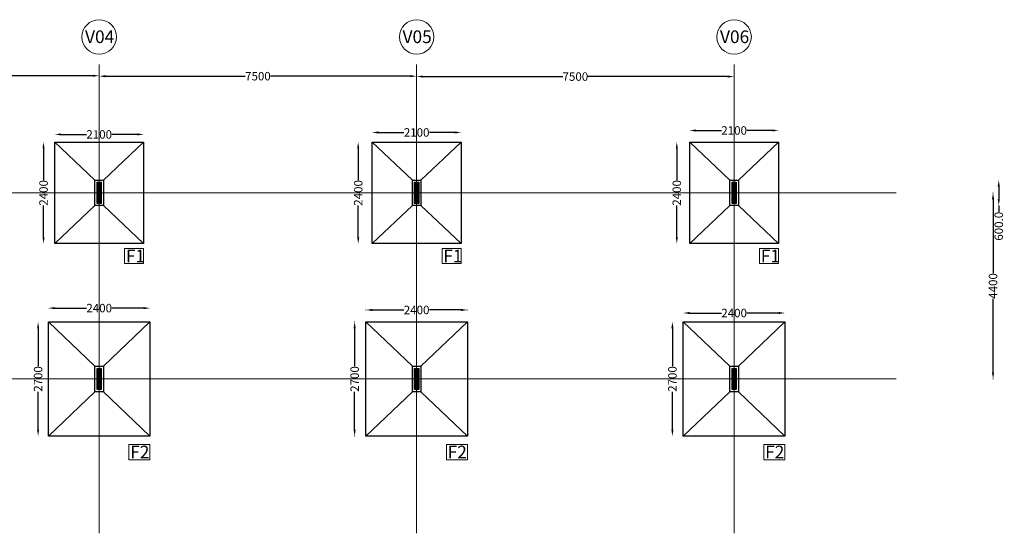
# Model space of a CAD drawing. Units: millimetres. Extents: x -30630 to 20484, y 3580 to 30715.
# Tile 4 of 4: x -3358 to 19903, y 16016 to 28161. Entities that reach past the tile are written whole.
import ezdxf

# ---------------------------------------------------------------- set-up
doc = ezdxf.new("R2010")
doc.units = ezdxf.units.MM
doc.header["$MEASUREMENT"] = 0
for name, color, linetype, lineweight in [('S-ANNO-DIMS', 2, 'Continuous', 18), ('S-ANNO-SYMB', 3, 'Continuous', 18), ('S-ANNO-TEXT', 7, 'Continuous', 18), ('S-FNDN', 7, 'Continuous', 30), ('S-GRID', 1, 'Continuous', 18), ('S-GRID-IDEN', 7, 'Continuous', 18)]:
    doc.layers.add(name, color=color, linetype=linetype, lineweight=lineweight)
doc.styles.get("Standard").update_dxf_attribs({"font": 'arial.ttf'})
doc.dimstyles.get("Standard").update_dxf_attribs({"dimtxt": 200, "dimasz": 150, "dimexe": 0.18, "dimexo": 0.0625, "dimgap": 0.09, "dimtad": 0, "dimdec": 0, "dimzin": 0, "dimdsep": 46, "dimtxsty": 'Standard', "dimcen": 0.09, "dimadec": 0, "dimazin": 0, "dimtfac": 1, "dimtdec": 0, "dimtofl": 0, "dimtmove": 0, "dimatfit": 3, "dimfxl": 1, "dimfxlon": 1, "dimtolj": 1, "dimtzin": 0, "dimarcsym": 0})

# ---------------------------------------------------------------- blocks, each defined once
blk = doc.blocks.new('*D5')
at = {"layer": 'Defpoints', "color": 0, "transparency": 16777216}
for p in [(-8980, 26835), (-8980, 26552), (-1480, 26552)]:
    blk.add_point(p, dxfattribs=at)
at = {"layer": 'S-ANNO-DIMS', "color": 0, "lineweight": -2, "transparency": 16777216}
for p, q in [((-8980, 26834), (-8980, 26836)), ((-8830, 26835), (-5528, 26835)), ((-1630, 26835), (-4933, 26835)), ((-1480, 26834), (-1480, 26836))]:
    blk.add_line(p, q, dxfattribs=at)
at = {"layer": 'S-ANNO-DIMS', "color": 0, "transparency": 16777216}
for points in [[(-8830, 26860), (-8830, 26810), (-8980, 26835)], [(-1630, 26860), (-1630, 26810), (-1480, 26835)]]:
    blk.add_solid(points, dxfattribs=at)
at = {"layer": 'S-ANNO-DIMS', "color": 0, "transparency": 16777216, "insert": (-5230, 26835), "char_height": 200, "attachment_point": 5}
blk.add_mtext('\\A1;7500', dxfattribs=at)
blk = doc.blocks.new('*D6')
at = {"layer": 'Defpoints', "color": 0, "transparency": 16777216}
for p in [(-1480, 26825), (-1480, 26456), (6020, 26456)]:
    blk.add_point(p, dxfattribs=at)
at = {"layer": 'S-ANNO-DIMS', "color": 0, "lineweight": -2, "transparency": 16777216}
for p, q in [((-1480, 26824), (-1480, 26825)), ((-1330, 26825), (1972, 26825)), ((5870, 26825), (2567, 26825)), ((6020, 26824), (6020, 26825))]:
    blk.add_line(p, q, dxfattribs=at)
at = {"layer": 'S-ANNO-DIMS', "color": 0, "transparency": 16777216}
for points in [[(-1330, 26850), (-1330, 26800), (-1480, 26825)], [(5870, 26850), (5870, 26800), (6020, 26825)]]:
    blk.add_solid(points, dxfattribs=at)
at = {"layer": 'S-ANNO-DIMS', "color": 0, "transparency": 16777216, "insert": (2270, 26825), "char_height": 200, "attachment_point": 5}
blk.add_mtext('\\A1;7500', dxfattribs=at)
blk = doc.blocks.new('*D7')
at = {"layer": 'Defpoints', "color": 0, "transparency": 16777216}
for p in [(6020, 26816), (6020, 26492), (13520, 26492)]:
    blk.add_point(p, dxfattribs=at)
at = {"layer": 'S-ANNO-DIMS', "color": 0, "lineweight": -2, "transparency": 16777216}
for p, q in [((6020, 26815), (6020, 26816)), ((6170, 26816), (9472, 26816)), ((13370, 26816), (10067, 26816)), ((13520, 26815), (13520, 26816))]:
    blk.add_line(p, q, dxfattribs=at)
at = {"layer": 'S-ANNO-DIMS', "color": 0, "transparency": 16777216}
for points in [[(6170, 26841), (6170, 26791), (6020, 26816)], [(13370, 26841), (13370, 26791), (13520, 26816)]]:
    blk.add_solid(points, dxfattribs=at)
at = {"layer": 'S-ANNO-DIMS', "color": 0, "transparency": 16777216, "insert": (9770, 26816), "char_height": 200, "attachment_point": 5}
blk.add_mtext('\\A1;7500', dxfattribs=at)
blk = doc.blocks.new('*D14')
at = {"layer": 'Defpoints', "color": 0, "transparency": 16777216}
for p in [(-2530, 25448), (-2530, 25265), (-430, 25265)]:
    blk.add_point(p, dxfattribs=at)
at = {"layer": 'S-ANNO-DIMS', "color": 0, "lineweight": -2, "transparency": 16777216}
for p, q in [((-2530, 25447), (-2530, 25448)), ((-2380, 25448), (-1780, 25448)), ((-580, 25448), (-1180, 25448)), ((-430, 25447), (-430, 25448))]:
    blk.add_line(p, q, dxfattribs=at)
at = {"layer": 'S-ANNO-DIMS', "color": 0, "transparency": 16777216}
for points in [[(-2380, 25473), (-2380, 25423), (-2530, 25448)], [(-580, 25473), (-580, 25423), (-430, 25448)]]:
    blk.add_solid(points, dxfattribs=at)
at = {"layer": 'S-ANNO-DIMS', "color": 0, "transparency": 16777216, "insert": (-1480, 25448), "char_height": 200, "attachment_point": 5}
blk.add_mtext('\\A1;2100', dxfattribs=at)
blk = doc.blocks.new('*D15')
at = {"layer": 'Defpoints', "color": 0, "transparency": 16777216}
for p in [(-2530, 25265), (-2795, 22865), (-2530, 22865)]:
    blk.add_point(p, dxfattribs=at)
at = {"layer": 'S-ANNO-DIMS', "color": 0, "lineweight": -2, "transparency": 16777216}
for p, q in [((-2794, 25265), (-2795, 25265)), ((-2795, 25115), (-2795, 24365)), ((-2795, 23015), (-2795, 23765)), ((-2794, 22865), (-2795, 22865))]:
    blk.add_line(p, q, dxfattribs=at)
at = {"layer": 'S-ANNO-DIMS', "color": 0, "transparency": 16777216}
for points in [[(-2820, 25115), (-2770, 25115), (-2795, 25265)], [(-2820, 23015), (-2770, 23015), (-2795, 22865)]]:
    blk.add_solid(points, dxfattribs=at)
at = {"layer": 'S-ANNO-DIMS', "color": 0, "transparency": 16777216, "insert": (-2795, 24065), "char_height": 200, "attachment_point": 5, "rotation": 90}
blk.add_mtext('\\A1;2400', dxfattribs=at)
blk = doc.blocks.new('*D16')
at = {"layer": 'Defpoints', "color": 0, "transparency": 16777216}
for p in [(7070, 25494), (4970, 25265), (7070, 25265)]:
    blk.add_point(p, dxfattribs=at)
at = {"layer": 'S-ANNO-DIMS', "color": 0, "lineweight": -2, "transparency": 16777216}
for p, q in [((4970, 25493), (4970, 25495)), ((5120, 25494), (5720, 25494)), ((6920, 25494), (6320, 25494)), ((7070, 25493), (7070, 25495))]:
    blk.add_line(p, q, dxfattribs=at)
at = {"layer": 'S-ANNO-DIMS', "color": 0, "transparency": 16777216}
for points in [[(5120, 25519), (5120, 25469), (4970, 25494)], [(6920, 25519), (6920, 25469), (7070, 25494)]]:
    blk.add_solid(points, dxfattribs=at)
at = {"layer": 'S-ANNO-DIMS', "color": 0, "transparency": 16777216, "insert": (6020, 25494), "char_height": 200, "attachment_point": 5}
blk.add_mtext('\\A1;2100', dxfattribs=at)
blk = doc.blocks.new('*D17')
at = {"layer": 'Defpoints', "color": 0, "transparency": 16777216}
for p in [(4970, 25265), (4639, 22865), (4970, 22865)]:
    blk.add_point(p, dxfattribs=at)
at = {"layer": 'S-ANNO-DIMS', "color": 0, "lineweight": -2, "transparency": 16777216}
for p, q in [((4640, 25265), (4639, 25265)), ((4639, 25115), (4639, 24365)), ((4639, 23015), (4639, 23765)), ((4640, 22865), (4639, 22865))]:
    blk.add_line(p, q, dxfattribs=at)
at = {"layer": 'S-ANNO-DIMS', "color": 0, "transparency": 16777216}
for points in [[(4614, 25115), (4664, 25115), (4639, 25265)], [(4614, 23015), (4664, 23015), (4639, 22865)]]:
    blk.add_solid(points, dxfattribs=at)
at = {"layer": 'S-ANNO-DIMS', "color": 0, "transparency": 16777216, "insert": (4639, 24065), "char_height": 200, "attachment_point": 5, "rotation": 90}
blk.add_mtext('\\A1;2400', dxfattribs=at)
blk = doc.blocks.new('*D18')
at = {"layer": 'Defpoints', "color": 0, "transparency": 16777216}
for p in [(12470, 25541), (12470, 25265), (14570, 25265)]:
    blk.add_point(p, dxfattribs=at)
at = {"layer": 'S-ANNO-DIMS', "color": 0, "lineweight": -2, "transparency": 16777216}
for p, q in [((12470, 25540), (12470, 25542)), ((12620, 25541), (13220, 25541)), ((14420, 25541), (13820, 25541)), ((14570, 25540), (14570, 25542))]:
    blk.add_line(p, q, dxfattribs=at)
at = {"layer": 'S-ANNO-DIMS', "color": 0, "transparency": 16777216}
for points in [[(12620, 25566), (12620, 25516), (12470, 25541)], [(14420, 25566), (14420, 25516), (14570, 25541)]]:
    blk.add_solid(points, dxfattribs=at)
at = {"layer": 'S-ANNO-DIMS', "color": 0, "transparency": 16777216, "insert": (13520, 25541), "char_height": 200, "attachment_point": 5}
blk.add_mtext('\\A1;2100', dxfattribs=at)
blk = doc.blocks.new('*D19')
at = {"layer": 'Defpoints', "color": 0, "transparency": 16777216}
for p in [(12470, 25265), (12166, 22865), (12470, 22865)]:
    blk.add_point(p, dxfattribs=at)
at = {"layer": 'S-ANNO-DIMS', "color": 0, "lineweight": -2, "transparency": 16777216}
for p, q in [((12167, 25265), (12166, 25265)), ((12166, 25115), (12166, 24365)), ((12166, 23015), (12166, 23765)), ((12167, 22865), (12166, 22865))]:
    blk.add_line(p, q, dxfattribs=at)
at = {"layer": 'S-ANNO-DIMS', "color": 0, "transparency": 16777216}
for points in [[(12141, 25115), (12191, 25115), (12166, 25265)], [(12141, 23015), (12191, 23015), (12166, 22865)]]:
    blk.add_solid(points, dxfattribs=at)
at = {"layer": 'S-ANNO-DIMS', "color": 0, "transparency": 16777216, "insert": (12166, 24065), "char_height": 200, "attachment_point": 5, "rotation": 90}
blk.add_mtext('\\A1;2400', dxfattribs=at)
blk = doc.blocks.new('*D26')
at = {"layer": 'Defpoints', "color": 0, "transparency": 16777216}
for p in [(-2680, 21341), (-2680, 21015), (-280, 21015)]:
    blk.add_point(p, dxfattribs=at)
at = {"layer": 'S-ANNO-DIMS', "color": 0, "lineweight": -2, "transparency": 16777216}
for p, q in [((-2680, 21340), (-2680, 21341)), ((-2530, 21341), (-1780, 21341)), ((-430, 21341), (-1180, 21341)), ((-280, 21340), (-280, 21341))]:
    blk.add_line(p, q, dxfattribs=at)
at = {"layer": 'S-ANNO-DIMS', "color": 0, "transparency": 16777216}
for points in [[(-2530, 21366), (-2530, 21316), (-2680, 21341)], [(-430, 21366), (-430, 21316), (-280, 21341)]]:
    blk.add_solid(points, dxfattribs=at)
at = {"layer": 'S-ANNO-DIMS', "color": 0, "transparency": 16777216, "insert": (-1480, 21341), "char_height": 200, "attachment_point": 5}
blk.add_mtext('\\A1;2400', dxfattribs=at)
blk = doc.blocks.new('*D27')
at = {"layer": 'Defpoints', "color": 0, "transparency": 16777216}
for p in [(-2680, 21015), (-2923, 18315), (-2680, 18315)]:
    blk.add_point(p, dxfattribs=at)
at = {"layer": 'S-ANNO-DIMS', "color": 0, "lineweight": -2, "transparency": 16777216}
for p, q in [((-2922, 21015), (-2923, 21015)), ((-2923, 20865), (-2923, 19965)), ((-2923, 18465), (-2923, 19365)), ((-2922, 18315), (-2923, 18315))]:
    blk.add_line(p, q, dxfattribs=at)
at = {"layer": 'S-ANNO-DIMS', "color": 0, "transparency": 16777216}
for points in [[(-2948, 20865), (-2898, 20865), (-2923, 21015)], [(-2948, 18465), (-2898, 18465), (-2923, 18315)]]:
    blk.add_solid(points, dxfattribs=at)
at = {"layer": 'S-ANNO-DIMS', "color": 0, "transparency": 16777216, "insert": (-2923, 19665), "char_height": 200, "attachment_point": 5, "rotation": 90}
blk.add_mtext('\\A1;2700', dxfattribs=at)
blk = doc.blocks.new('*D28')
at = {"layer": 'Defpoints', "color": 0, "transparency": 16777216}
for p in [(4820, 21297), (4820, 21015), (7220, 21015)]:
    blk.add_point(p, dxfattribs=at)
at = {"layer": 'S-ANNO-DIMS', "color": 0, "lineweight": -2, "transparency": 16777216}
for p, q in [((4820, 21296), (4820, 21298)), ((4970, 21297), (5720, 21297)), ((7070, 21297), (6320, 21297)), ((7220, 21296), (7220, 21298))]:
    blk.add_line(p, q, dxfattribs=at)
at = {"layer": 'S-ANNO-DIMS', "color": 0, "transparency": 16777216}
for points in [[(4970, 21322), (4970, 21272), (4820, 21297)], [(7070, 21322), (7070, 21272), (7220, 21297)]]:
    blk.add_solid(points, dxfattribs=at)
at = {"layer": 'S-ANNO-DIMS', "color": 0, "transparency": 16777216, "insert": (6020, 21297), "char_height": 200, "attachment_point": 5}
blk.add_mtext('\\A1;2400', dxfattribs=at)
blk = doc.blocks.new('*D29')
at = {"layer": 'Defpoints', "color": 0, "transparency": 16777216}
for p in [(4820, 21015), (4555, 18315), (4820, 18315)]:
    blk.add_point(p, dxfattribs=at)
at = {"layer": 'S-ANNO-DIMS', "color": 0, "lineweight": -2, "transparency": 16777216}
for p, q in [((4556, 21015), (4555, 21015)), ((4555, 20865), (4555, 19965)), ((4555, 18465), (4555, 19365)), ((4556, 18315), (4555, 18315))]:
    blk.add_line(p, q, dxfattribs=at)
at = {"layer": 'S-ANNO-DIMS', "color": 0, "transparency": 16777216}
for points in [[(4530, 20865), (4580, 20865), (4555, 21015)], [(4530, 18465), (4580, 18465), (4555, 18315)]]:
    blk.add_solid(points, dxfattribs=at)
at = {"layer": 'S-ANNO-DIMS', "color": 0, "transparency": 16777216, "insert": (4555, 19665), "char_height": 200, "attachment_point": 5, "rotation": 90}
blk.add_mtext('\\A1;2700', dxfattribs=at)
blk = doc.blocks.new('*D30')
at = {"layer": 'Defpoints', "color": 0, "transparency": 16777216}
for p in [(12320, 21225), (12320, 21015), (14720, 21015)]:
    blk.add_point(p, dxfattribs=at)
at = {"layer": 'S-ANNO-DIMS', "color": 0, "lineweight": -2, "transparency": 16777216}
for p, q in [((12320, 21224), (12320, 21225)), ((12470, 21225), (13220, 21225)), ((14570, 21225), (13820, 21225)), ((14720, 21224), (14720, 21225))]:
    blk.add_line(p, q, dxfattribs=at)
at = {"layer": 'S-ANNO-DIMS', "color": 0, "transparency": 16777216}
for points in [[(12470, 21250), (12470, 21200), (12320, 21225)], [(14570, 21250), (14570, 21200), (14720, 21225)]]:
    blk.add_solid(points, dxfattribs=at)
at = {"layer": 'S-ANNO-DIMS', "color": 0, "transparency": 16777216, "insert": (13520, 21225), "char_height": 200, "attachment_point": 5}
blk.add_mtext('\\A1;2400', dxfattribs=at)
blk = doc.blocks.new('*D31')
at = {"layer": 'Defpoints', "color": 0, "transparency": 16777216}
for p in [(12320, 21015), (12062, 18315), (12320, 18315)]:
    blk.add_point(p, dxfattribs=at)
at = {"layer": 'S-ANNO-DIMS', "color": 0, "lineweight": -2, "transparency": 16777216}
for p, q in [((12063, 21015), (12062, 21015)), ((12062, 20865), (12062, 19965)), ((12062, 18465), (12062, 19365)), ((12063, 18315), (12062, 18315))]:
    blk.add_line(p, q, dxfattribs=at)
at = {"layer": 'S-ANNO-DIMS', "color": 0, "transparency": 16777216}
for points in [[(12037, 20865), (12087, 20865), (12062, 21015)], [(12037, 18465), (12087, 18465), (12062, 18315)]]:
    blk.add_solid(points, dxfattribs=at)
at = {"layer": 'S-ANNO-DIMS', "color": 0, "transparency": 16777216, "insert": (12062, 19665), "char_height": 200, "attachment_point": 5, "rotation": 90}
blk.add_mtext('\\A1;2700', dxfattribs=at)
blk = doc.blocks.new('FOOTING-F1')
h = blk.add_hatch()
h.set_pattern_fill('ANSI31', color=256, scale=100)
h.set_pattern_definition([(45, (50626.339, 2179.544), (-8.8388348, 8.8388348), [])])
h.paths.add_polyline_path([(1100, 24315), (1000, 24315), (1000, 23815), (1100, 23815)])
for p, q in [((0, 25265), (950, 24365)), ((1150, 24365), (2100, 25265)), ((950, 23765), (0, 22865)), ((1150, 23765), (2100, 22865))]:
    blk.add_line(p, q)
for points in [[(0, 25265), (2100, 25265), (2100, 22865), (0, 22865)], [(950, 24365), (1150, 24365), (1150, 23765), (950, 23765)], [(1000, 24315), (1100, 24315), (1100, 23815), (1000, 23815)]]:
    blk.add_lwpolyline(points, close=True)
blk = doc.blocks.new('FOOTING-F2')
h = blk.add_hatch()
h.set_pattern_fill('ANSI31', color=256, scale=100)
h.set_pattern_definition([(45, (58801.161, 2265.705), (-8.8388348, 8.8388348), [])])
h.paths.add_polyline_path([(1250, 19915), (1150, 19915), (1150, 19415), (1250, 19415)])
for p, q in [((1100, 19965), (0, 21015)), ((1300, 19965), (2400, 21015)), ((1100, 19365), (0, 18315)), ((1300, 19365), (2400, 18315))]:
    blk.add_line(p, q)
for points in [[(0, 21015), (2400, 21015), (2400, 18315), (0, 18315)], [(1100, 19965), (1300, 19965), (1300, 19365), (1100, 19365)], [(1150, 19915), (1250, 19915), (1250, 19415), (1150, 19415)]]:
    blk.add_lwpolyline(points, close=True)
blk = doc.blocks.new('*D35')
at = {"layer": 'Defpoints', "color": 0, "transparency": 16777216}
for p in [(17349.335413, 24064.719518), (17349.335413, 19664.719518), (19636.835413, 19664.719518)]:
    blk.add_point(p, dxfattribs=at)
at = {"layer": 'S-ANNO-DIMS', "color": 0, "lineweight": -2, "transparency": 16777216}
for p, q in [((19635.835413, 24064.719518), (19637.015413, 24064.719518)), ((19636.835413, 23914.719518), (19636.835413, 22167.128754)), ((19636.835413, 19814.719518), (19636.835413, 21562.310282)), ((19635.835413, 19664.719518), (19637.015413, 19664.719518))]:
    blk.add_line(p, q, dxfattribs=at)
at = {"layer": 'S-ANNO-DIMS', "color": 0, "transparency": 16777216}
for points in [[(19611.835413, 23914.719518), (19661.835413, 23914.719518), (19636.835413, 24064.719518)], [(19611.835413, 19814.719518), (19661.835413, 19814.719518), (19636.835413, 19664.719518)]]:
    blk.add_solid(points, dxfattribs=at)
at = {"layer": 'S-ANNO-DIMS', "color": 0, "transparency": 16777216, "insert": (19636.835413, 21864.719518), "char_height": 200, "attachment_point": 5, "rotation": 90}
blk.add_mtext('\\A1;4400', dxfattribs=at)
blk = doc.blocks.new('*D65')
at = {"layer": 'Defpoints', "color": 0, "transparency": 16777216}
for p in [(-23880, 24365), (-23880, 23765), (19772, 23765)]:
    blk.add_point(p, dxfattribs=at)
at = {"layer": 'S-ANNO-DIMS', "color": 0, "lineweight": -2, "transparency": 16777216}
for p, q in [((19771, 24365), (19772, 24365)), ((19772, 24215), (19772, 23915)), ((19771, 23765), (19772, 23765)), ((19772, 23765), (19772, 23615))]:
    blk.add_line(p, q, dxfattribs=at)
at = {"layer": 'S-ANNO-DIMS', "color": 0, "transparency": 16777216}
for points in [[(19747, 24215), (19797, 24215), (19772, 24365)], [(19747, 23915), (19797, 23915), (19772, 23765)]]:
    blk.add_solid(points, dxfattribs=at)
at = {"layer": 'S-ANNO-DIMS', "color": 0, "transparency": 16777216, "insert": (19772, 23277), "char_height": 200, "attachment_point": 5, "rotation": 90}
blk.add_mtext('\\A1;600.0', dxfattribs=at)

msp = doc.modelspace()

# ---------------------------------------------------------------- linework, layer by layer
at = {"layer": 'S-ANNO-SYMB'}
for points in [[(-880.1095, 22391.7904), (-880.1095, 22753.0183), (-430.0685, 22753.0183), (-430.0685, 22391.7904)], [(6619.8905, 22391.7904), (6619.8905, 22753.0183), (7069.9315, 22753.0183), (7069.9315, 22391.7904)], [(14119.8905, 22391.7904), (14119.8905, 22753.0183), (14569.9315, 22753.0183), (14569.9315, 22391.7904)], [(-777.1763, 17757.175), (-777.1763, 18118.4029), (-280.0685, 18118.4029), (-280.0685, 17757.175)], [(6722.8237, 17757.175), (6722.8237, 18118.4029), (7219.9315, 18118.4029), (7219.9315, 17757.175)], [(14222.8237, 17757.175), (14222.8237, 18118.4029), (14719.9315, 18118.4029), (14719.9315, 17757.175)]]:
    msp.add_lwpolyline(points, close=True, dxfattribs=at)
at = {"layer": 'S-GRID'}
for p, q in [((-1480.0685, 27102.0571), (-1480.0685, 16015.6561)), ((6019.9315, 27102.0571), (6019.9315, 16015.6561)), ((13519.9315, 27102.0571), (13519.9315, 16015.6561)), ((-26695.8159, 24064.7195), (17349.3354, 24064.7195)), ((-26695.8159, 19664.7195), (17349.3354, 19664.7195))]:
    msp.add_line(p, q, dxfattribs=at)
at = {"layer": 'S-GRID-IDEN'}
for centre in [(-1480.0685, 27753.8802), (6019.9315, 27753.8802), (13519.9315, 27753.8802)]:
    msp.add_circle(centre, 407.0061, dxfattribs=at)

# ---------------------------------------------------------------- block references
at = {"layer": 'S-FNDN'}
for name, p in [('FOOTING-F1', (-2530.069, 0)), ('FOOTING-F1', (4969.931, 0)), ('FOOTING-F1', (12469.931, 0)), ('FOOTING-F2', (-2680.069, 0)), ('FOOTING-F2', (4819.931, 0)), ('FOOTING-F2', (12319.931, 0))]:
    msp.add_blockref(name, p, dxfattribs=at)

# ---------------------------------------------------------------- texts
at = {"layer": 'S-ANNO-TEXT', "char_height": 300, "attachment_point": 1}
for s, width, insert in [('V04', 4876.019723, (-1813.5269, 27907.0521)), ('V05', 4876.019723, (5686.4731, 27907.0521)), ('V06', 4876.019723, (13186.4731, 27907.0521)), ('{\\fArial|b1|i0|c0|p34;F1}', 1058.385802, (-850.1095, 22723.0183)), ('{\\fArial|b1|i0|c0|p34;F1}', 1058.385802, (6649.8905, 22723.0183)), ('{\\fArial|b1|i0|c0|p34;F1}', 1058.385802, (14149.8905, 22723.0183)), ('{\\fArial|b1|i0|c0|p34;F2}', 1058.385802, (-747.1763, 18088.4029)), ('{\\fArial|b1|i0|c0|p34;F2}', 1058.385802, (6752.8237, 18088.4029)), ('{\\fArial|b1|i0|c0|p34;F2}', 1058.385802, (14252.8237, 18088.4029))]:
    msp.add_mtext_dynamic_manual_height_columns(s, width=width, gutter_width=1, heights=[0], dxfattribs=dict(at, insert=insert))

# ---------------------------------------------------------------- dimensions: what is measured, and where the dimension line sits
at = {"layer": 'S-ANNO-DIMS'}
for base, p1, p2, picture, middle in [((-8980.0685, 26835.3937), (-1480.0685, 26552.1998), (-8980.0685, 26552.1998), '*D5', (-5230.0685, 26835.3937)), ((-1480.0685, 26825.1445), (6019.9315, 26456.1747), (-1480.0685, 26456.1747), '*D6', (2269.9315, 26825.1445)), ((6019.9315, 26816.1351), (13519.9315, 26491.794), (6019.9315, 26491.794), '*D7', (9769.9315, 26816.1351)), ((7069.9315, 25494.4318), (4969.9315, 25264.7195), (7069.9315, 25264.7195), '*D16', (6019.9315, 25494.4318)), ((12469.9315, 25541.4655), (14569.9315, 25264.7195), (12469.9315, 25264.7195), '*D18', (13519.9315, 25541.4655)), ((-2530.0685, 25447.8625), (-430.0685, 25264.7195), (-2530.0685, 25264.7195), '*D14', (-1480.0685, 25447.8625)), ((-2680.0685, 21340.9924), (-280.0685, 21014.7195), (-2680.0685, 21014.7195), '*D26', (-1480.0685, 21340.9924)), ((4819.9315, 21297.42), (7219.9315, 21014.7195), (4819.9315, 21014.7195), '*D28', (6019.9315, 21297.42)), ((12319.9315, 21224.8698), (14719.9315, 21014.7195), (12319.9315, 21014.7195), '*D30', (13519.9315, 21224.8698))]:
    dim = msp.add_linear_dim(base=base, p1=p1, p2=p2, dimstyle='Standard', override={"dimclrd": 0, "dimclre": 0, "dimclrt": 0}, dxfattribs=at)
    dim.commit()
    dim.dimension.update_dxf_attribs({"geometry": picture, "text_midpoint": middle})
for base, p1, p2, override, picture, middle in [((-2794.744, 22864.7195), (-2530.0685, 25264.7195), (-2530.0685, 22864.7195), {"dimclrd": 0, "dimclre": 0, "dimclrt": 0}, '*D15', (-2794.744, 24064.7195)), ((4638.7734, 22864.7195), (4969.9315, 25264.7195), (4969.9315, 22864.7195), {"dimclrd": 0, "dimclre": 0, "dimclrt": 0}, '*D17', (4638.7734, 24064.7195)), ((12165.8759, 22864.7195), (12469.9315, 25264.7195), (12469.9315, 22864.7195), {"dimclrd": 0, "dimclre": 0, "dimclrt": 0}, '*D19', (12165.8759, 24064.7195)), ((19771.8354, 23764.7195), (-23880.0685, 24364.7195), (-23880.0685, 23764.7195), {"dimdec": 1, "dimlfac": 1, "dimrnd": 0, "dimzin": 0, "dimdsep": 46, "dimlunit": 2}, '*D65', (19771.8354, 23276.976)), ((19636.8354, 19664.7195), (17349.3354, 24064.7195), (17349.3354, 19664.7195), {"dimdec": 0, "dimlfac": 1, "dimrnd": 0, "dimzin": 0, "dimdsep": 46, "dimlunit": 2}, '*D35', (19636.8354, 21864.7195)), ((-2923.2347, 18314.7195), (-2680.0685, 21014.7195), (-2680.0685, 18314.7195), {"dimclrd": 0, "dimclre": 0, "dimclrt": 0}, '*D27', (-2923.2347, 19664.7195)), ((4555.4248, 18314.7195), (4819.9315, 21014.7195), (4819.9315, 18314.7195), {"dimclrd": 0, "dimclre": 0, "dimclrt": 0}, '*D29', (4555.4248, 19664.7195)), ((12061.82, 18314.7195), (12319.9315, 21014.7195), (12319.9315, 18314.7195), {"dimclrd": 0, "dimclre": 0, "dimclrt": 0}, '*D31', (12061.82, 19664.7195))]:
    dim = msp.add_linear_dim(base=base, p1=p1, p2=p2, angle=90, dimstyle='Standard', override=override, dxfattribs=at)
    dim.commit()
    dim.dimension.update_dxf_attribs({"geometry": picture, "text_midpoint": middle})

doc.saveas('drawing.dxf')
